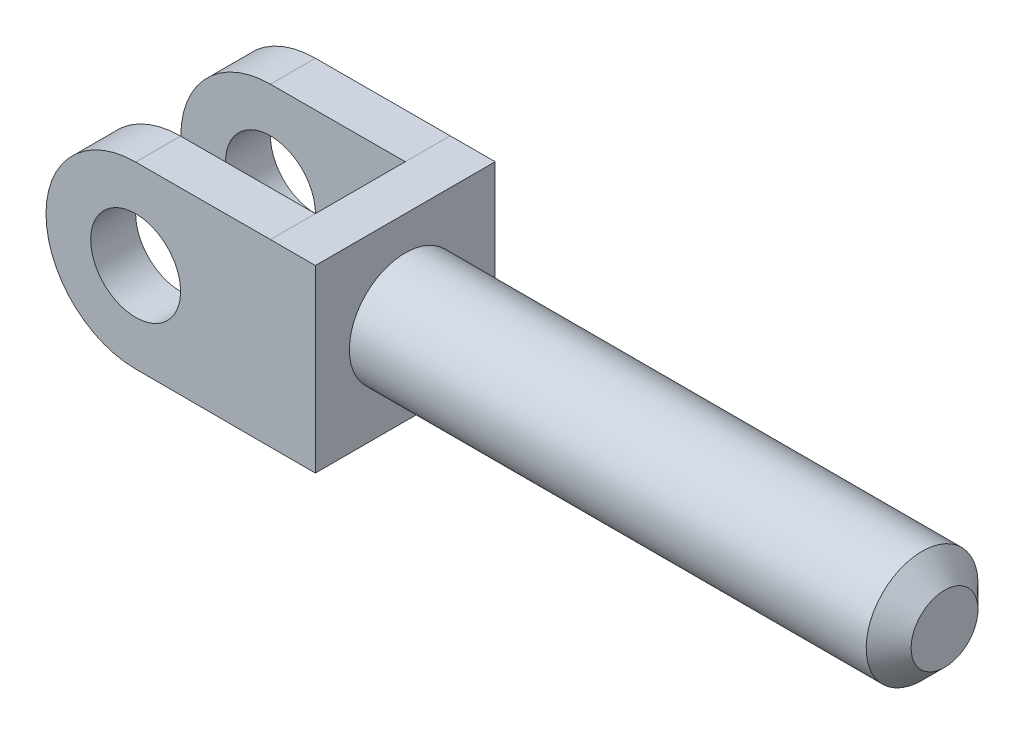
from build123d import *

# Parameters (mm, degrees)
CLEVIS_BLOCK_SKETCH_W  = 3.175
CLEVIS_BLOCK_SKETCH_H  = 12.7
CLEVIS_BLOCK_DEPTH     = 6.35
SHANK_SKETCH_7_95_R    = 3.95
SHANK_7_95_DEPTH       = 38.1
SHANK_END_CHAMFER_SIZE = 1.5875
CLEVIS_EAR_SKETCH_R    = 3.175
CLEVIS_EAR_DEPTH       = 3.175


with BuildPart() as part:
    # Clevis Block Sketch → Clevis Block (new, symmetric)
    with BuildSketch(Plane.XY):
        with Locations((1.5875, 0)):
            Rectangle(CLEVIS_BLOCK_SKETCH_W, CLEVIS_BLOCK_SKETCH_H)
    extrude(amount=CLEVIS_BLOCK_DEPTH, both=True)

    # Shank Sketch Ø7.95 → Shank Ø7.95 (add)
    with BuildSketch(Plane(origin=(3.175, 0, 0), x_dir=(0, 0, -1), z_dir=(1, 0, 0))):
        with Locations(Location((0, 0, 0), (0, 0, 270))):
            Circle(SHANK_SKETCH_7_95_R)
    extrude(amount=SHANK_7_95_DEPTH)

    # Shank End Chamfer
    shank_end_chamfer_edges = [part.edges().sort_by_distance(p)[0] for p in [
        (41.275, 3.95, 0),
    ]]
    chamfer(shank_end_chamfer_edges, length=SHANK_END_CHAMFER_SIZE)

    # Clevis Ear Sketch → Clevis Ear (add)
    with BuildSketch(Plane(origin=(0, 0, -6.35), x_dir=(-1, 0, 0), z_dir=(0, 0, -1))):
        with BuildLine():
            Line((9.525, 6.332334812), (0, 6.35))
            Line((0, 6.35), (0, -6.35))
            Line((0, -6.35), (9.525, -6.332334812))
            ThreePointArc((9.525, -6.332334812), (15.857334812, 0), (9.525, 6.332334812))
        make_face()
        with Locations((9.525, 0)):
            Circle(CLEVIS_EAR_SKETCH_R, mode=Mode.SUBTRACT)
    clevis_ear = extrude(amount=-CLEVIS_EAR_DEPTH)

    # Clevis Ear Mirror: Clevis Ear across plane
    add(clevis_ear.mirror(Plane.XY))


solid = part.part
